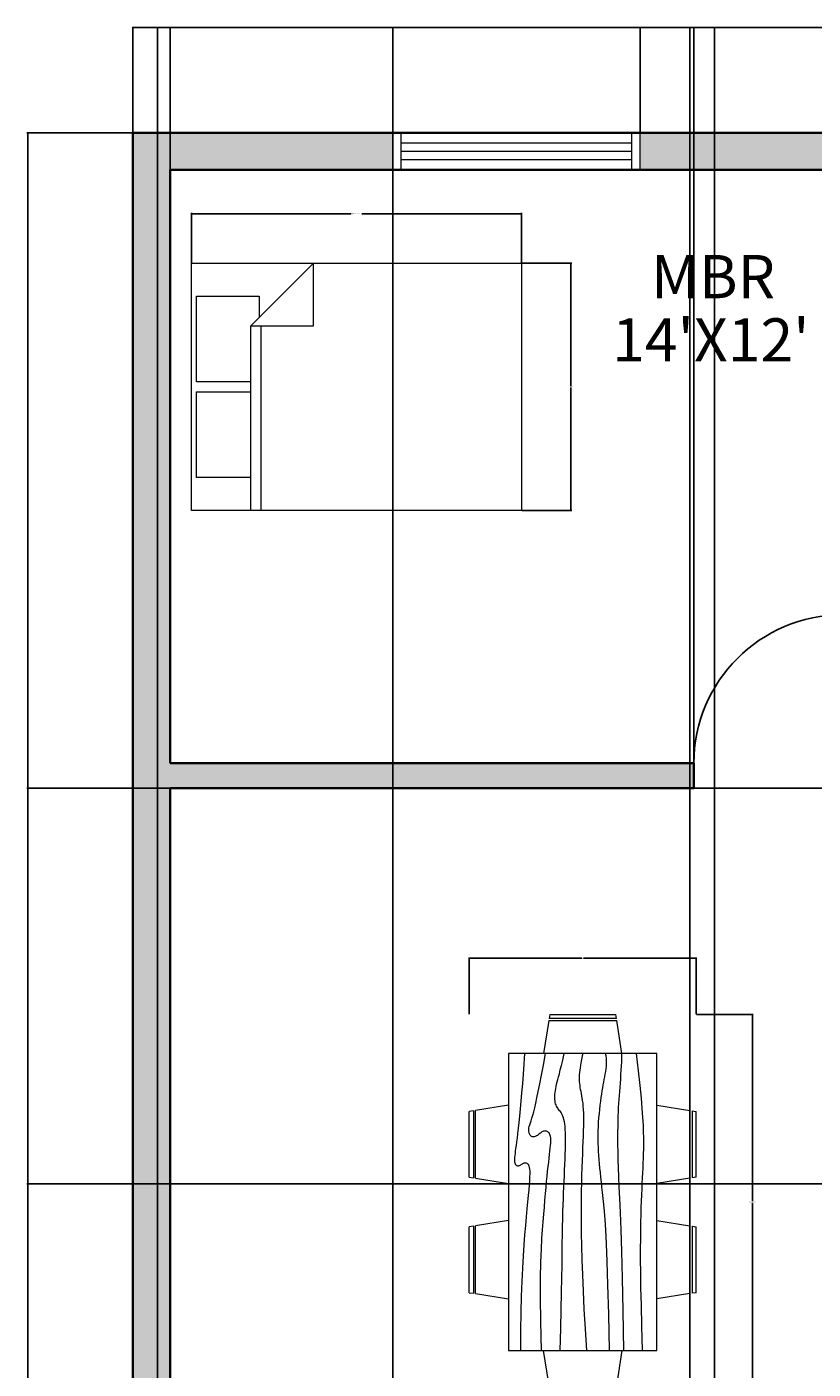
# Model space of a CAD drawing. Units: inches. Extents: x -82 to 330, y 553 to 1115.
# Tile 3 of 4: x -82 to 109, y 789 to 1115. Entities that reach past the tile are written whole.
import ezdxf

# ---------------------------------------------------------------- set-up
doc = ezdxf.new("R2010")
doc.units = ezdxf.units.IN
for name, color, linetype, lineweight in [('A-ANNO-DIMS', 2, 'Continuous', 18), ('A-AREA-IDEN', 7, 'Continuous', 25), ('A-DOOR', 3, 'Continuous', 25), ('A-FURN', 8, 'Continuous', 18), ('A-GLAZ', 4, 'Continuous', 18), ('A-WALL', 7, 'Continuous', 35)]:
    doc.layers.add(name, color=color, linetype=linetype, lineweight=lineweight)
doc.layers.add('A-WALL-PATT', color=18, linetype='Continuous', lineweight=13, true_color=0x000000)
doc.styles.get("Standard").update_dxf_attribs({"font": 'arial.ttf'})
doc.dimstyles.get("Standard").update_dxf_attribs({"dimtxt": 0.18, "dimasz": 0.18, "dimexe": 0.18, "dimexo": 0.0625, "dimgap": 0.09, "dimtad": 0, "dimtih": 1, "dimtoh": 1, "dimdec": 4, "dimzin": 0, "dimdsep": 46, "dimtxsty": 'Standard', "dimcen": 0.09, "dimadec": 0, "dimazin": 0, "dimtfac": 1, "dimtdec": 4, "dimtofl": 0, "dimtmove": 0, "dimatfit": 3, "dimfxl": 1, "dimtolj": 1, "dimtzin": 0, "dimarcsym": 0})

# ---------------------------------------------------------------- blocks, each defined once
blk = doc.blocks.new('Dining Set - 36 x 72 in.')
for p, q in [((-22, 27.5), (-22.1562, 26.50042)), ((-5.8416, 26.5), (-22.1534, 26.5)), ((-22, 27.5), (-6, 27.5)), ((-5.8437, 26.49966), (-6, 27.5)), ((6, 27.5), (5.8438, 26.50042)), ((22.1584, 26.5), (5.8466, 26.5)), ((6, 27.5), (22, 27.5)), ((22.1563, 26.49966), (22, 27.5)), ((-22.2343, 26.00059), (-23.4847, 17.99762)), ((-22.2304, 26), (-5.7608, 26)), ((-4.5152, 17.99762), (-5.7655, 25.99926)), ((5.7657, 26.00059), (4.5153, 17.99762)), ((5.7696, 26), (22.2392, 26)), ((23.4848, 17.99762), (22.2345, 25.99926)), ((36, 18), (-36, 18)), ((-36, 18), (-36, -18)), ((36, -18), (36, 18)), ((-45.5, 8), (-44.5004, 8.15617)), ((-45.5, 8), (-45.5, -8)), ((-44.5, -8.15843), (-44.5, 8.15338)), ((-44.0006, 8.23428), (-35.9976, 9.48474)), ((-44, 8.23041), (-44, -8.23915)), ((44.0006, 8.23428), (35.9976, 9.48474)), ((44, 8.23041), (44, -8.23915)), ((44.5, -8.15843), (44.5, 8.15338)), ((45.5, 8), (44.5005, 8.15617)), ((45.5, 8), (45.5, -8)), ((-44.4997, -8.15631), (-45.5, -8)), ((-35.9976, -9.48476), (-43.9993, -8.2345)), ((35.9976, -9.48476), (43.9993, -8.2345)), ((44.4997, -8.15631), (45.5, -8)), ((-36, -18), (36, -18)), ((-22.2343, -26.0006), (-23.4847, -17.99762)), ((-4.5152, -17.99762), (-5.7655, -25.99928)), ((5.7657, -26.0006), (4.5153, -17.99762)), ((23.4848, -17.99762), (22.2345, -25.99928)), ((-22.2304, -26), (-5.7608, -26)), ((5.7696, -26), (22.2392, -26)), ((-22, -27.5), (-22.1562, -26.50044)), ((-5.8416, -26.5), (-22.1534, -26.5)), ((-22, -27.5), (-6, -27.5)), ((-5.8437, -26.49967), (-6, -27.5)), ((6, -27.5), (5.8438, -26.50044)), ((22.1584, -26.5), (5.8466, -26.5)), ((6, -27.5), (22, -27.5)), ((22.1563, -26.49967), (22, -27.5))]:
    blk.add_line(p, q)
for points in [[(-36, 15), (-31.1772, 14.97754), (-26.8079, 14.91406), (-22.8538, 14.81543), (-19.276, 14.6875), (-16.0362, 14.53613), (-13.0957, 14.36718), (-10.4159, 14.18652), (-7.9583, 14), (-5.6904, 13.81315), (-3.6035, 13.63021), (-1.6954, 13.45508), (0.0365, 13.29166), (1.5945, 13.14388), (2.9811, 13.01562), (4.1988, 12.9108), (5.25, 12.83333), (6.1393, 12.78613), (6.8802, 12.76823), (7.4883, 12.77767), (7.9792, 12.8125), (8.3685, 12.87077), (8.6719, 12.95052), (8.9049, 13.0498), (9.0833, 13.16666), (9.2205, 13.29899), (9.3216, 13.44401), (9.3895, 13.59879), (9.4271, 13.76041), (9.4373, 13.92594), (9.4232, 14.09245), (9.3875, 14.257), (9.3333, 14.41666), (9.2638, 14.56917), (9.1836, 14.71484), (9.0975, 14.85465), (9.0104, 14.98958), (8.9272, 15.1206), (8.8529, 15.2487), (8.7922, 15.37483), (8.75, 15.5), (8.7305, 15.62467), (8.7344, 15.74739), (8.7617, 15.86621), (8.8125, 15.97916), (8.8867, 16.08431), (8.9844, 16.17968), (9.1055, 16.26334), (9.25, 16.33333), (9.4189, 16.38802), (9.6172, 16.42708), (9.8506, 16.45052), (10.125, 16.45833), (10.4463, 16.45052), (10.8203, 16.42708), (11.2529, 16.38802), (11.75, 16.33333), (12.3184, 16.26318), (12.9694, 16.17838), (13.7151, 16.07991), (14.5677, 15.96875), (15.5395, 15.84586), (16.6426, 15.71224), (17.8893, 15.56884), (19.2917, 15.41666), (20.859, 15.25667), (22.5879, 15.08984), (24.4721, 14.91715), (26.5052, 14.73958), (28.6809, 14.5581), (30.9929, 14.3737), (33.4347, 14.18733), (36, 14)], [(-36, 10), (-28.9766, 10.14274), (-23.1725, 10.20442), (-18.4241, 10.19775), (-14.5677, 10.13541), (-11.4399, 10.03011), (-8.877, 9.89453), (-6.7154, 9.74137), (-4.7917, 9.58333), (-2.9698, 9.43082), (-1.2246, 9.28515), (0.4415, 9.14534), (2.026, 9.01041), (3.5266, 8.87939), (4.9408, 8.7513), (6.266, 8.62516), (7.5, 8.5), (8.6411, 8.37549), (9.6914, 8.2539), (10.6538, 8.13818), (11.5312, 8.03125), (12.3267, 7.93603), (13.043, 7.85547), (13.6831, 7.79248), (14.25, 7.75), (14.7471, 7.7303), (15.1797, 7.73307), (15.5537, 7.75732), (15.875, 7.80208), (16.1494, 7.86637), (16.3828, 7.94922), (16.5811, 8.04964), (16.75, 8.16666), (16.8944, 8.29915), (17.0143, 8.44531), (17.1089, 8.60319), (17.1771, 8.77083), (17.218, 8.94629), (17.2305, 9.1276), (17.2137, 9.31282), (17.1667, 9.5), (17.0895, 9.6875), (16.987, 9.875), (16.8649, 10.0625), (16.7292, 10.25), (16.5856, 10.4375), (16.4401, 10.625), (16.2985, 10.8125), (16.1667, 11), (16.05, 11.18733), (15.9518, 11.3737), (15.8752, 11.5581), (15.8229, 11.73958), (15.798, 11.91715), (15.8034, 12.08984), (15.842, 12.25667), (15.9167, 12.41666), (16.0295, 12.56836), (16.1784, 12.70833), (16.3605, 12.83268), (16.5729, 12.9375), (16.8127, 13.01888), (17.0768, 13.07291), (17.3625, 13.0957), (17.6667, 13.08333), (17.9894, 13.03312), (18.3418, 12.94726), (18.7382, 12.82918), (19.1927, 12.68229), (19.7195, 12.51001), (20.3327, 12.31575), (21.0465, 12.10294), (21.875, 11.875), (22.8357, 11.63354), (23.959, 11.37304), (25.2786, 11.08618), (26.8282, 10.76562), (28.6414, 10.40405), (30.752, 9.99414), (33.1936, 9.52856), (36, 9)], [(-36, 5.5), (-30.7157, 5.3348), (-26.069, 5.20963), (-21.9946, 5.11767), (-18.4271, 5.05208), (-15.3009, 5.00602), (-12.5508, 4.97265), (-10.1112, 4.94515), (-7.9167, 4.91666), (-5.909, 4.88167), (-4.0586, 4.83984), (-2.3429, 4.79215), (-0.7396, 4.73958), (0.7739, 4.6831), (2.22, 4.6237), (3.6213, 4.56233), (5, 4.5), (6.373, 4.43782), (7.7344, 4.3776), (9.0723, 4.32129), (10.375, 4.27083), (11.6309, 4.22819), (12.8281, 4.19531), (13.9551, 4.17415), (15, 4.16666), (15.954, 4.17448), (16.819, 4.19791), (17.6001, 4.23698), (18.3021, 4.29166), (18.9299, 4.36198), (19.4883, 4.44791), (19.9823, 4.54948), (20.4167, 4.66666), (20.7969, 4.79899), (21.1302, 4.94401), (21.4245, 5.09879), (21.6875, 5.26041), (21.9271, 5.42594), (22.1511, 5.59245), (22.3672, 5.757), (22.5834, 5.91666), (22.8065, 6.06868), (23.0404, 6.21093), (23.2879, 6.34147), (23.5521, 6.45833), (23.8358, 6.55957), (24.142, 6.64323), (24.4735, 6.70735), (24.8334, 6.75), (25.2235, 6.76969), (25.642, 6.76692), (26.0858, 6.74267), (26.5521, 6.69791), (27.0379, 6.63362), (27.5404, 6.55078), (28.0565, 6.45036), (28.5834, 6.33333), (29.1242, 6.19987), (29.7071, 6.04687), (30.3661, 5.87044), (31.1354, 5.66666), (32.0493, 5.43164), (33.142, 5.16146), (34.4475, 4.85221), (36, 4.5)], [(-36, -1), (-30.7915, -0.6591), (-26.0195, -0.38216), (-21.6519, -0.16284), (-17.6563, 0.00521), (-14.0005, 0.12833), (-10.6523, 0.21289), (-7.5796, 0.26522), (-4.75, 0.29166), (-2.134, 0.29793), (0.2878, 0.28711), (2.5317, 0.26163), (4.6146, 0.22396), (6.5529, 0.17651), (8.3633, 0.12174), (10.0623, 0.06209), (11.6667, 0), (13.1899, -0.06201), (14.6341, -0.1211), (15.9982, -0.17432), (17.2813, -0.21875), (18.4823, -0.25147), (19.6003, -0.26953), (20.6343, -0.27002), (21.5834, -0.25), (22.4481, -0.20768), (23.2357, -0.14584), (23.9549, -0.06836), (24.6146, 0.02083), (25.2235, 0.11784), (25.7904, 0.21875), (26.3241, 0.31966), (26.8334, 0.41666), (27.3265, 0.50618), (27.8099, 0.58593), (28.2894, 0.65397), (28.7709, 0.70833), (29.2601, 0.74707), (29.763, 0.76823), (30.2855, 0.76985), (30.8334, 0.75), (31.4088, 0.70784), (31.9994, 0.64713), (32.589, 0.57275), (33.1615, 0.48958), (33.7008, 0.4025), (34.1908, 0.3164), (34.6153, 0.23616), (34.9584, 0.16666), (35.2099, 0.11165), (35.3848, 0.07031), (35.504, 0.04069), (35.5886, 0.02083), (35.6594, 0.00879), (35.7377, 0.0026), (35.8442, 0.00032), (36, 0)], [(-36, -6.5), (-27.1843, -6.31267), (-20.084, -6.1263), (-14.469, -5.9419), (-10.1094, -5.76042), (-6.7752, -5.58285), (-4.2363, -5.41016), (-2.2629, -5.24333), (-0.625, -5.08334), (0.8708, -4.93099), (2.2715, -4.78646), (3.5872, -4.64974), (4.8281, -4.52084), (6.0046, -4.39974), (7.127, -4.28646), (8.2053, -4.18099), (9.25, -4.08334), (10.2705, -3.99382), (11.2734, -3.91407), (12.2647, -3.84603), (13.25, -3.79167), (14.2354, -3.75293), (15.2266, -3.73177), (16.2295, -3.73015), (17.25, -3.75), (18.2912, -3.79248), (19.3451, -3.85547), (20.4009, -3.93604), (21.4479, -4.03125), (22.4754, -4.13819), (23.4727, -4.25391), (24.4289, -4.37549), (25.3334, -4.5), (26.1785, -4.62492), (26.9694, -4.74935), (27.7145, -4.87281), (28.4219, -4.99479), (29.1, -5.11483), (29.7572, -5.23242), (30.4016, -5.34709), (31.0417, -5.45834), (31.6837, -5.56437), (32.3262, -5.65821), (32.9658, -5.73153), (33.599, -5.77604), (34.2224, -5.78345), (34.8327, -5.74545), (35.4264, -5.65373), (36, -5.5)], [(-36, -10), (-26.4022, -9.81299), (-18.4675, -9.62891), (-11.9839, -9.45069), (-6.7396, -9.28125), (-2.5226, -9.12354), (0.8789, -8.98047), (3.6769, -8.85498), (6.0833, -8.75), (8.2767, -8.66765), (10.3021, -8.60677), (12.1712, -8.56543), (13.8958, -8.54167), (15.4876, -8.53353), (16.9583, -8.53907), (18.3197, -8.55632), (19.5834, -8.58334), (20.7616, -8.61841), (21.8685, -8.66081), (22.9188, -8.71004), (23.9271, -8.76563), (24.9081, -8.82707), (25.8763, -8.89388), (26.8465, -8.96558), (27.8334, -9.04167), (28.8474, -9.12118), (29.8828, -9.20117), (30.93, -9.27824), (31.9792, -9.34896), (33.0205, -9.40991), (34.0443, -9.45768), (35.0407, -9.48885), (36, -9.5)], [(-36, -14.5), (-30.0881, -14.33513), (-25.0332, -14.21224), (-20.7312, -14.12647), (-17.0781, -14.07292), (-13.97, -14.04671), (-11.3027, -14.04297), (-8.9724, -14.05681), (-6.875, -14.08334), (-4.9224, -14.11833), (-3.0905, -14.16016), (-1.3709, -14.20785), (0.2448, -14.26042), (1.7647, -14.3169), (3.1973, -14.3763), (4.5507, -14.43767), (5.8333, -14.5), (7.0554, -14.5621), (8.235, -14.62175), (9.3922, -14.67652), (10.5469, -14.72396), (11.7192, -14.76164), (12.929, -14.78711), (14.1965, -14.79794), (15.5417, -14.79167), (16.9933, -14.76424), (18.6152, -14.70508), (20.4804, -14.60197), (22.6615, -14.44271), (25.2312, -14.21509), (28.2624, -13.9069), (31.8277, -13.50594), (36, -13)]]:
    blk.add_lwpolyline(points)
blk = doc.blocks.new('Bed - Queen')
for p, q in [((0, -80.00003), (0, 0)), ((0, 0), (59.99999, 0)), ((59.99999, 0), (59.99999, -80.00003)), ((7.99999, -1.2), (28.79998, -1.2)), ((7.99999, -14.4), (7.99999, -1.2)), ((28.79998, -1.2), (28.79998, -14.4)), ((31.19999, -1.2), (51.99999, -1.2)), ((31.19999, -14.4), (31.19999, -1.2)), ((51.99999, -1.2), (51.99999, -16.4)), ((0, -14.4), (44.8, -14.4)), ((59.99999, -29.6), (44.8, -14.4)), ((44.8, -14.4), (44.8, -29.6)), ((44.8, -16.8), (0, -16.8)), ((51.99999, -16.4), (46.79936, -16.4)), ((44.8, -29.6), (59.99999, -29.6)), ((59.99999, -80.00003), (0, -80.00003))]:
    blk.add_line(p, q)
blk = doc.blocks.new('WIN-60IN')
for p, q in [((60, 9), (0, 9)), ((0, 9), (0, 0)), ((2, 9), (2, 0)), ((58, 0), (58, 9)), ((60, 0), (60, 9)), ((2, 6.5), (58, 6.5)), ((2, 4.5), (58, 4.5)), ((0, 0), (60, 0)), ((2, 2.5), (58, 2.5))]:
    blk.add_line(p, q)
blk = doc.blocks.new('DOOR-SWING-36IN')
for p, q in [((0, 36), (0, 0)), ((3, 36), (3, 0)), ((0, 0), (3, 0))]:
    blk.add_line(p, q)
blk.add_arc((0, 0), 36, 0, 90)
blk = doc.blocks.new('*D15')
at = {"layer": 'A-ANNO-DIMS', "color": 0, "lineweight": -2, "transparency": 16777216}
for p, q in [((-41.8, 1057.52), (-41.8, 1069.64)), ((-41.62, 1069.46), (-3.1, 1069.46)), ((38.02, 1069.46), (-0.5, 1069.46)), ((38.2, 1057.52), (38.2, 1069.64))]:
    blk.add_line(p, q, dxfattribs=at)
at = {"layer": 'A-ANNO-DIMS', "color": 0, "transparency": 16777216}
for points in [[(-41.62, 1069.49), (-41.62, 1069.43), (-41.8, 1069.46)], [(38.02, 1069.49), (38.02, 1069.43), (38.2, 1069.46)]]:
    blk.add_solid(points, dxfattribs=at)
at = {"layer": 'Defpoints', "color": 0, "transparency": 16777216}
for p in [(-41.8, 1069.46), (-41.8, 1057.46), (38.2, 1057.46)]:
    blk.add_point(p, dxfattribs=at)
at = {"layer": 'A-ANNO-DIMS', "color": 0, "transparency": 16777216, "insert": (-1.8, 1069.46), "char_height": 0.18, "attachment_point": 5}
blk.add_mtext('\\A1;QUEEN BED 80 TYP.', dxfattribs=at)
blk = doc.blocks.new('*D16')
at = {"layer": 'A-ANNO-DIMS', "color": 0, "lineweight": -2, "transparency": 16777216}
for p, q in [((38.26, 1057.46), (50.38, 1057.46)), ((50.2, 1057.28), (50.2, 1027.64)), ((50.2, 997.64), (50.2, 1027.28)), ((38.26, 997.46), (50.38, 997.46))]:
    blk.add_line(p, q, dxfattribs=at)
at = {"layer": 'A-ANNO-DIMS', "color": 0, "transparency": 16777216}
for points in [[(50.17, 1057.28), (50.23, 1057.28), (50.2, 1057.46)], [(50.17, 997.64), (50.23, 997.64), (50.2, 997.46)]]:
    blk.add_solid(points, dxfattribs=at)
at = {"layer": 'Defpoints', "color": 0, "transparency": 16777216}
for p in [(38.2, 1057.46), (50.2, 1057.46), (38.2, 997.46)]:
    blk.add_point(p, dxfattribs=at)
at = {"layer": 'A-ANNO-DIMS', "color": 0, "transparency": 16777216, "insert": (50.2, 1027.46), "char_height": 0.18, "attachment_point": 5}
blk.add_mtext('\\A1;60 TYP.', dxfattribs=at)
blk = doc.blocks.new('*D27')
at = {"layer": 'A-ANNO-DIMS', "color": 0, "lineweight": -2, "transparency": 16777216}
for p, q in [((80.61, 875.16), (94.38, 875.16)), ((94.2, 874.98), (94.2, 829.85)), ((94.2, 784.34), (94.2, 829.48)), ((80.61, 784.16), (94.38, 784.16))]:
    blk.add_line(p, q, dxfattribs=at)
at = {"layer": 'A-ANNO-DIMS', "color": 0, "transparency": 16777216}
for points in [[(94.17, 874.98), (94.23, 874.98), (94.2, 875.16)], [(94.17, 784.34), (94.23, 784.34), (94.2, 784.16)]]:
    blk.add_solid(points, dxfattribs=at)
at = {"layer": 'Defpoints', "color": 0, "transparency": 16777216}
for p in [(80.55, 875.16), (94.2, 875.16), (80.55, 784.16)]:
    blk.add_point(p, dxfattribs=at)
at = {"layer": 'A-ANNO-DIMS', "color": 0, "transparency": 16777216, "insert": (94.2, 829.66), "char_height": 0.18, "attachment_point": 5}
blk.add_mtext('\\A1;DINING SET 91', dxfattribs=at)
blk = doc.blocks.new('*D28')
at = {"layer": 'A-ANNO-DIMS', "color": 0, "lineweight": -2, "transparency": 16777216}
for p, q in [((25.55, 875.23), (25.55, 888.99)), ((25.73, 888.81), (52.83, 888.81)), ((80.37, 888.81), (53.27, 888.81)), ((80.55, 875.23), (80.55, 888.99))]:
    blk.add_line(p, q, dxfattribs=at)
at = {"layer": 'A-ANNO-DIMS', "color": 0, "transparency": 16777216}
for points in [[(25.73, 888.84), (25.73, 888.78), (25.55, 888.81)], [(80.37, 888.84), (80.37, 888.78), (80.55, 888.81)]]:
    blk.add_solid(points, dxfattribs=at)
at = {"layer": 'Defpoints', "color": 0, "transparency": 16777216}
for p in [(25.55, 888.81), (25.55, 875.16), (80.55, 875.16)]:
    blk.add_point(p, dxfattribs=at)
at = {"layer": 'A-ANNO-DIMS', "color": 0, "transparency": 16777216, "insert": (53.05, 888.81), "char_height": 0.18, "attachment_point": 5}
blk.add_mtext('\\A1;55', dxfattribs=at)
blk = doc.blocks.new('*D32')
at = {"layer": 'A-ANNO-DIMS', "color": 0, "lineweight": -2, "transparency": 16777216}
for p, q in [((-56.07, 1089.11), (-81.69, 1089.11)), ((-81.51, 1088.93), (-81.51, 834.29)), ((-81.51, 579.29), (-81.51, 833.93)), ((0.93, 579.11), (-81.69, 579.11))]:
    blk.add_line(p, q, dxfattribs=at)
at = {"layer": 'A-ANNO-DIMS', "color": 0, "transparency": 16777216}
for points in [[(-81.54, 1088.93), (-81.48, 1088.93), (-81.51, 1089.11)], [(-81.54, 579.29), (-81.48, 579.29), (-81.51, 579.11)]]:
    blk.add_solid(points, dxfattribs=at)
at = {"layer": 'Defpoints', "color": 0, "transparency": 16777216}
for p in [(-81.51, 1089.11), (-56.01, 1089.11), (0.99, 579.11)]:
    blk.add_point(p, dxfattribs=at)
at = {"layer": 'A-ANNO-DIMS', "color": 0, "transparency": 16777216, "insert": (-81.51, 834.11), "char_height": 0.18, "attachment_point": 5}
blk.add_mtext('\\A1;510', dxfattribs=at)
blk = doc.blocks.new('*D33')
at = {"layer": 'A-ANNO-DIMS', "color": 0, "lineweight": -2, "transparency": 16777216}
for p, q in [((-56.01, 1089.17), (-56.01, 1114.79)), ((-55.83, 1114.61), (-24.73, 1114.61)), ((6.81, 1114.61), (-24.29, 1114.61)), ((6.99, 1089.17), (6.99, 1114.79))]:
    blk.add_line(p, q, dxfattribs=at)
at = {"layer": 'A-ANNO-DIMS', "color": 0, "transparency": 16777216}
for points in [[(-55.83, 1114.64), (-55.83, 1114.58), (-56.01, 1114.61)], [(6.81, 1114.64), (6.81, 1114.58), (6.99, 1114.61)]]:
    blk.add_solid(points, dxfattribs=at)
at = {"layer": 'Defpoints', "color": 0, "transparency": 16777216}
for p in [(6.99, 1114.61), (-56.01, 1089.11), (6.99, 1089.11)]:
    blk.add_point(p, dxfattribs=at)
at = {"layer": 'A-ANNO-DIMS', "color": 0, "transparency": 16777216, "insert": (-24.51, 1114.61), "char_height": 0.18, "attachment_point": 5}
blk.add_mtext('\\A1;63', dxfattribs=at)
blk = doc.blocks.new('*D34')
at = {"layer": 'A-ANNO-DIMS', "color": 0, "lineweight": -2, "transparency": 16777216}
for p, q in [((66.99, 1089.17), (66.99, 1114.79)), ((67.17, 1114.61), (123.71, 1114.61)), ((180.81, 1114.61), (124.27, 1114.61)), ((180.99, 1089.17), (180.99, 1114.79))]:
    blk.add_line(p, q, dxfattribs=at)
at = {"layer": 'A-ANNO-DIMS', "color": 0, "transparency": 16777216}
for points in [[(67.17, 1114.64), (67.17, 1114.58), (66.99, 1114.61)], [(180.81, 1114.64), (180.81, 1114.58), (180.99, 1114.61)]]:
    blk.add_solid(points, dxfattribs=at)
at = {"layer": 'Defpoints', "color": 0, "transparency": 16777216}
for p in [(180.99, 1114.61), (66.99, 1089.11), (180.99, 1089.11)]:
    blk.add_point(p, dxfattribs=at)
at = {"layer": 'A-ANNO-DIMS', "color": 0, "transparency": 16777216, "insert": (123.99, 1114.61), "char_height": 0.18, "attachment_point": 5}
blk.add_mtext('\\A1;114', dxfattribs=at)
blk = doc.blocks.new('*D35')
at = {"layer": 'A-ANNO-DIMS', "color": 0, "lineweight": -2, "transparency": 16777216}
for p, q in [((84.99, 627.17), (84.99, 1114.79)), ((85.17, 1114.61), (110.29, 1114.61)), ((135.81, 1114.61), (110.69, 1114.61)), ((135.99, 618.17), (135.99, 1114.79))]:
    blk.add_line(p, q, dxfattribs=at)
at = {"layer": 'A-ANNO-DIMS', "color": 0, "transparency": 16777216}
for points in [[(85.17, 1114.64), (85.17, 1114.58), (84.99, 1114.61)], [(135.81, 1114.64), (135.81, 1114.58), (135.99, 1114.61)]]:
    blk.add_solid(points, dxfattribs=at)
at = {"layer": 'Defpoints', "color": 0, "transparency": 16777216}
for p in [(135.99, 1114.61), (84.99, 627.11), (135.99, 618.11)]:
    blk.add_point(p, dxfattribs=at)
at = {"layer": 'A-ANNO-DIMS', "color": 0, "transparency": 16777216, "insert": (110.49, 1114.61), "char_height": 0.18, "attachment_point": 5}
blk.add_mtext('\\A1;51', dxfattribs=at)
blk = doc.blocks.new('*D36')
at = {"layer": 'A-ANNO-DIMS', "color": 0, "lineweight": -2, "transparency": 16777216}
for p, q in [((6.99, 627.17), (6.99, 1114.79)), ((7.17, 1114.61), (42.77, 1114.61)), ((78.81, 1114.61), (43.21, 1114.61)), ((78.99, 627.17), (78.99, 1114.79))]:
    blk.add_line(p, q, dxfattribs=at)
at = {"layer": 'A-ANNO-DIMS', "color": 0, "transparency": 16777216}
for points in [[(7.17, 1114.64), (7.17, 1114.58), (6.99, 1114.61)], [(78.81, 1114.64), (78.81, 1114.58), (78.99, 1114.61)]]:
    blk.add_solid(points, dxfattribs=at)
at = {"layer": 'Defpoints', "color": 0, "transparency": 16777216}
for p in [(78.99, 1114.61), (6.99, 627.11), (78.99, 627.11)]:
    blk.add_point(p, dxfattribs=at)
at = {"layer": 'A-ANNO-DIMS', "color": 0, "transparency": 16777216, "insert": (42.99, 1114.61), "char_height": 0.18, "attachment_point": 5}
blk.add_mtext('\\A1;72', dxfattribs=at)
blk = doc.blocks.new('*D45')
at = {"layer": 'A-ANNO-DIMS', "color": 0, "lineweight": -2, "transparency": 16777216}
for p, q in [((180.93, 930.11), (-81.69, 930.11)), ((-81.51, 929.93), (-81.51, 882.29)), ((-81.51, 834.29), (-81.51, 881.93)), ((180.93, 834.11), (-81.69, 834.11))]:
    blk.add_line(p, q, dxfattribs=at)
at = {"layer": 'A-ANNO-DIMS', "color": 0, "transparency": 16777216}
for points in [[(-81.54, 929.93), (-81.48, 929.93), (-81.51, 930.11)], [(-81.54, 834.29), (-81.48, 834.29), (-81.51, 834.11)]]:
    blk.add_solid(points, dxfattribs=at)
at = {"layer": 'Defpoints', "color": 0, "transparency": 16777216}
for p in [(180.99, 930.11), (-81.51, 834.11), (180.99, 834.11)]:
    blk.add_point(p, dxfattribs=at)
at = {"layer": 'A-ANNO-DIMS', "color": 0, "transparency": 16777216, "insert": (-81.51, 882.11), "char_height": 0.18, "attachment_point": 5}
blk.add_mtext('\\A1;96', dxfattribs=at)
blk = doc.blocks.new('*D46')
at = {"layer": 'A-ANNO-DIMS', "color": 0, "lineweight": -2, "transparency": 16777216}
for p, q in [((-47.01, 936.17), (-47.01, 1114.79)), ((-46.83, 1114.61), (16.21, 1114.61)), ((79.81, 1114.61), (16.77, 1114.61)), ((79.99, 936.17), (79.99, 1114.79))]:
    blk.add_line(p, q, dxfattribs=at)
at = {"layer": 'A-ANNO-DIMS', "color": 0, "transparency": 16777216}
for points in [[(-46.83, 1114.64), (-46.83, 1114.58), (-47.01, 1114.61)], [(79.81, 1114.64), (79.81, 1114.58), (79.99, 1114.61)]]:
    blk.add_solid(points, dxfattribs=at)
at = {"layer": 'Defpoints', "color": 0, "transparency": 16777216}
for p in [(79.99, 1114.61), (-47.01, 936.11), (79.99, 936.11)]:
    blk.add_point(p, dxfattribs=at)
at = {"layer": 'A-ANNO-DIMS', "color": 0, "transparency": 16777216, "insert": (16.49, 1114.61), "char_height": 0.18, "attachment_point": 5}
blk.add_mtext('\\A1;127', dxfattribs=at)
blk = doc.blocks.new('*D48')
at = {"layer": 'A-ANNO-DIMS', "color": 0, "lineweight": -2, "transparency": 16777216}
for p, q in [((-50.01, 609.17), (-50.01, 1114.79)), ((-49.83, 1114.61), (42.71, 1114.61)), ((135.81, 1114.61), (43.27, 1114.61)), ((135.99, 618.17), (135.99, 1114.79))]:
    blk.add_line(p, q, dxfattribs=at)
at = {"layer": 'A-ANNO-DIMS', "color": 0, "transparency": 16777216}
for points in [[(-49.83, 1114.64), (-49.83, 1114.58), (-50.01, 1114.61)], [(135.81, 1114.64), (135.81, 1114.58), (135.99, 1114.61)]]:
    blk.add_solid(points, dxfattribs=at)
at = {"layer": 'Defpoints', "color": 0, "transparency": 16777216}
for p in [(135.99, 1114.61), (135.99, 618.11), (-50.01, 609.11)]:
    blk.add_point(p, dxfattribs=at)
at = {"layer": 'A-ANNO-DIMS', "color": 0, "transparency": 16777216, "insert": (42.99, 1114.61), "char_height": 0.18, "attachment_point": 5}
blk.add_mtext('\\A1;186', dxfattribs=at)

msp = doc.modelspace()

# ---------------------------------------------------------------- hatches: boundary and pattern name
at = {"layer": 'A-WALL-PATT'}
h = msp.add_hatch(color=256, dxfattribs=at)
h.dxf.hatch_style = 1
h.paths.add_polyline_path([(6.988, 1089.11), (-56.012, 1089.11), (-56.012, 705.11), (-47.012, 705.11), (-15.012, 705.11), (-15.012, 714.11), (-47.012, 714.11), (-47.012, 930.11), (79.988, 930.11), (79.988, 936.11), (-47.012, 936.11), (-47.012, 1080.11), (6.988, 1080.11)])
h.paths.add_polyline_path([(180.988, 1089.11), (66.988, 1089.11), (66.988, 1080.11), (120.988, 1080.11), (120.988, 936.11), (115.988, 936.11), (115.988, 930.11), (131.988, 930.11), (131.988, 936.11), (126.988, 936.11), (126.988, 1080.11), (180.988, 1080.11)])
h.paths.add_polyline_path([(303.988, 1089.11), (240.988, 1089.11), (240.988, 1080.11), (294.988, 1080.11), (294.988, 936.11), (167.988, 936.11), (167.988, 930.11), (180.988, 930.11), (180.988, 834.11), (186.988, 834.11), (186.988, 930.11), (294.988, 930.11), (294.988, 867.11), (303.988, 867.11)])
h.paths.add_polyline_path([(303.988, 855.11), (294.988, 855.11), (294.988, 792.11), (186.988, 792.11), (186.988, 804.11), (180.988, 804.11), (180.988, 792.11), (144.988, 792.11), (144.988, 756.11), (150.988, 756.11), (150.988, 786.11), (294.988, 786.11), (294.988, 732.11), (303.988, 732.11)])
h.paths.add_polyline_path([(303.988, 672.11), (294.988, 672.11), (294.988, 618.11), (150.988, 618.11), (150.988, 720.11), (144.988, 720.11), (144.988, 714.11), (124.988, 714.11), (124.988, 705.11), (144.988, 705.11), (144.988, 618.11), (144.988, 609.11), (303.988, 609.11)])
h.paths.add_polyline_path([(76.988, 714.11), (44.988, 714.11), (44.988, 705.11), (76.988, 705.11)], flags=17)
h = msp.add_hatch(color=256, dxfattribs=at)
h.dxf.hatch_style = 1
h.paths.add_polyline_path([(-50.012, 615.11), (-56.012, 615.11), (-56.012, 609.11), (-50.012, 609.11)])
h.paths.add_polyline_path([(144.988, 615.11), (135.988, 615.11), (135.988, 609.11), (144.988, 609.11)])
h.paths.add_polyline_path([(-47.012, 930.11), (79.988, 930.11), (79.988, 936.11), (-47.012, 936.11), (-47.012, 1080.11), (6.988, 1080.11), (6.988, 1089.11), (-56.012, 1089.11), (-56.012, 705.11), (-47.012, 705.11), (-15.012, 705.11), (-15.012, 714.11), (-47.012, 714.11)])

# ---------------------------------------------------------------- linework, layer by layer
at = {"layer": 'A-WALL'}
for p, q in [((303.988, 1089.11), (-56.012, 1089.11)), ((-56.012, 1089.11), (-56.012, 609.11)), ((-47.012, 1080.11), (-47.012, 936.11)), ((120.988, 1080.11), (-47.012, 1080.11)), ((79.988, 936.11), (-47.012, 936.11)), ((79.988, 936.11), (79.988, 930.11)), ((79.988, 930.11), (-47.012, 930.11)), ((-47.012, 930.11), (-47.012, 714.11))]:
    msp.add_line(p, q, dxfattribs=at)

# ---------------------------------------------------------------- block references
at = {"layer": 'A-DOOR', "extrusion": (0, 0, -1), "zscale": -1}
msp.add_blockref('DOOR-SWING-36IN', (-115.989, 936.11), dxfattribs=at)
at = {"layer": 'A-FURN', "rotation": 90}
for name, p in [('Bed - Queen', (-41.799, 997.462)), ('Dining Set - 36 x 72 in.', (53.047, 829.664))]:
    msp.add_blockref(name, p, dxfattribs=at)
at = {"layer": 'A-GLAZ'}
msp.add_blockref('WIN-60IN', (6.988, 1080.11), dxfattribs=at)

# ---------------------------------------------------------------- texts
at = {"layer": 'A-AREA-IDEN', "char_height": 10.4756, "attachment_point": 1}
for s, insert in [('MBR', (69.605, 1059.424)), ("14'X12'", (60.187, 1044.072))]:
    msp.add_mtext_dynamic_manual_height_columns(s, width=470.55254, gutter_width=52.378, heights=[0], dxfattribs=dict(at, insert=insert))

# ---------------------------------------------------------------- dimensions: what is measured, and where the dimension line sits
at = {"layer": 'A-ANNO-DIMS'}
for base, p1, p2, picture, middle in [((6.988, 1114.611), (-56.012, 1089.11), (6.988, 1089.11), '*D33', (-24.512, 1114.611)), ((135.988, 1114.611), (-50.012, 609.11), (135.988, 618.11), '*D48', (42.988, 1114.611)), ((79.988, 1114.611), (-47.012, 936.11), (79.988, 936.11), '*D46', (16.488, 1114.611)), ((78.988, 1114.611), (6.988, 627.11), (78.988, 627.11), '*D36', (42.988, 1114.611)), ((180.988, 1114.611), (66.988, 1089.11), (180.988, 1089.11), '*D34', (123.988, 1114.611)), ((135.988, 1114.611), (84.988, 627.11), (135.988, 618.11), '*D35', (110.488, 1114.611))]:
    dim = msp.add_linear_dim(base=base, p1=p1, p2=p2, dimstyle='Standard', override={"dimdec": 0, "dimlfac": 1, "dimrnd": 0, "dimzin": 0, "dimdsep": 46, "dimlunit": 2}, dxfattribs=at)
    dim.commit()
    dim.dimension.update_dxf_attribs({"geometry": picture, "text_midpoint": middle})
for base, p1, p2, angle, picture, middle in [((-81.513, 1089.11), (0.988, 579.11), (-56.012, 1089.11), 90, '*D32', (-81.513, 834.11)), ((-81.513, 834.11), (180.988, 930.11), (180.988, 834.11), 90, '*D45', (-81.513, 882.11)), ((25.547, 888.814), (80.547, 875.164), (25.547, 875.164), 180, '*D28', (53.047, 888.814))]:
    dim = msp.add_linear_dim(base=base, p1=p1, p2=p2, angle=angle, dimstyle='Standard', override={"dimdec": 0, "dimlfac": 1, "dimrnd": 0, "dimzin": 0, "dimdsep": 46, "dimlunit": 2}, dxfattribs=at)
    dim.commit()
    dim.dimension.update_dxf_attribs({"geometry": picture, "text_midpoint": middle})
for base, p1, p2, angle, text, picture, middle in [((-41.799, 1069.462), (38.201, 1057.462), (-41.799, 1057.462), 180, 'QUEEN BED <> TYP.', '*D15', (-1.799, 1069.462)), ((50.201, 1057.462), (38.201, 997.462), (38.201, 1057.462), 90, '<> TYP.', '*D16', (50.201, 1027.462)), ((94.197, 875.164), (80.547, 784.164), (80.547, 875.164), 90, 'DINING SET <>', '*D27', (94.197, 829.664))]:
    dim = msp.add_linear_dim(base=base, p1=p1, p2=p2, angle=angle, text=text, dimstyle='Standard', override={"dimdec": 0, "dimlfac": 1, "dimrnd": 0, "dimzin": 0, "dimdsep": 46, "dimlunit": 2}, dxfattribs=at)
    dim.commit()
    dim.dimension.update_dxf_attribs({"geometry": picture, "text_midpoint": middle})

doc.saveas('drawing.dxf')
